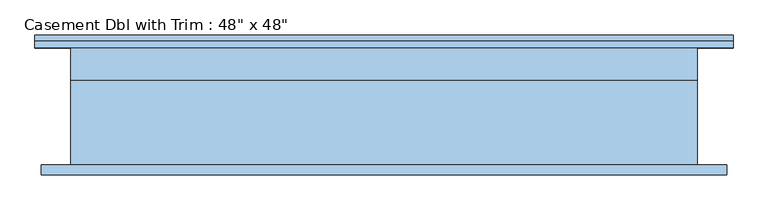
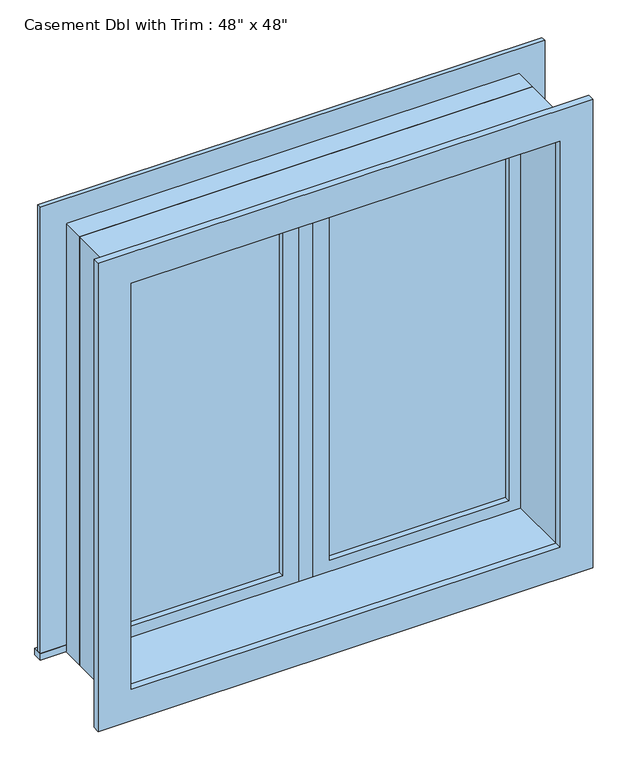
"""IFC4 building model written with IfcOpenShell, lengths in millimetres: window geometry."""

from ifc_helpers import new_model, si_unit, frame, origin, place, context, project, spatial, polyline, outline, extrude, source, transform, mapped, element, save


def window_534dcd48(model_context):
    return source(origin(), model_context, "Body", "SweptSolid", [
        extrude(outline(polyline([(63.5, 98.425), (546.1, 98.425), (546.1, 85.725), (63.5, 85.725), (63.5, 98.425)])), frame((0.0, 0.0, 977.9), z_axis=(0.0, 0.0, 1.0), x_axis=(1.0, 0.0, 0.0)), (0.0, 0.0, 1.0), 1092.2),
        extrude(outline(polyline([(2114.55, 19.05), (933.45, 19.05), (933.45, 590.55), (2114.55, 590.55), (2114.55, 19.05)]), holes=[polyline([(2070.1, 63.5), (2070.1, 546.1), (977.9, 546.1), (977.9, 63.5), (2070.1, 63.5)])]), frame((0.0, 69.85, 0.0), z_axis=(0.0, 1.0, 0.0), x_axis=(0.0, 0.0, 1.0)), (0.0, 0.0, 1.0), 44.45),
        extrude(outline(polyline([(19.05, 69.85), (-19.05, 69.85), (-19.05, 133.35), (19.05, 133.35), (19.05, 69.85)])), frame((0.0, 0.0, 933.45), z_axis=(0.0, 0.0, 1.0), x_axis=(1.0, 0.0, 0.0)), (0.0, 0.0, 1.0), 1181.1),
        extrude(outline(polyline([(-679.45, 158.75), (679.45, 158.75), (679.45, 133.35), (-679.45, 133.35), (-679.45, 158.75)])), frame((0.0, 0.0, 914.4), z_axis=(0.0, 0.0, 1.0), x_axis=(1.0, 0.0, 0.0)), (0.0, 0.0, 1.0), 19.05),
        extrude(outline(polyline([(2114.55, -590.55), (2114.55, 590.55), (933.45, 590.55), (933.45, 679.45), (2203.45, 679.45), (2203.45, -679.45), (933.45, -679.45), (933.45, -590.55), (2114.55, -590.55)])), frame((0.0, 133.35, 0.0), z_axis=(0.0, 1.0, 0.0), x_axis=(0.0, 0.0, 1.0)), (0.0, 0.0, 1.0), 12.7),
        extrude(outline(polyline([(2190.75, 666.75), (2190.75, -666.75), (857.25, -666.75), (857.25, 666.75), (2190.75, 666.75)]), holes=[polyline([(2101.85, 577.85), (946.15, 577.85), (946.15, -577.85), (2101.85, -577.85), (2101.85, 577.85)])]), frame((0.0, -114.3, 0.0), z_axis=(0.0, 1.0, 0.0), x_axis=(0.0, 0.0, 1.0)), (0.0, 0.0, 1.0), 19.05),
        extrude(outline(polyline([(-63.5, 85.725), (-546.1, 85.725), (-546.1, 98.425), (-63.5, 98.425), (-63.5, 85.725)])), frame((0.0, 0.0, 977.9), z_axis=(0.0, 0.0, 1.0), x_axis=(1.0, 0.0, 0.0)), (0.0, 0.0, 1.0), 1092.2),
        extrude(outline(polyline([(2114.55, -590.55), (933.45, -590.55), (933.45, -19.05), (2114.55, -19.05), (2114.55, -590.55)]), holes=[polyline([(2070.1, -546.1), (2070.1, -63.5), (977.9, -63.5), (977.9, -546.1), (2070.1, -546.1)])]), frame((0.0, 69.85, 0.0), z_axis=(0.0, 1.0, 0.0), x_axis=(0.0, 0.0, 1.0)), (0.0, 0.0, 1.0), 44.45),
        extrude(outline(polyline([(2133.6, -609.6), (914.4, -609.6), (914.4, 609.6), (2133.6, 609.6), (2133.6, -609.6)]), holes=[polyline([(2101.85, -577.85), (2101.85, 577.85), (946.15, 577.85), (946.15, -577.85), (2101.85, -577.85)])]), frame((0.0, -95.25, 0.0), z_axis=(0.0, 1.0, 0.0), x_axis=(0.0, 0.0, 1.0)), (0.0, 0.0, 1.0), 165.1),
        extrude(outline(polyline([(2133.6, 609.6), (2133.6, -609.6), (914.4, -609.6), (914.4, 609.6), (2133.6, 609.6)]), holes=[polyline([(2114.55, 590.55), (933.45, 590.55), (933.45, -590.55), (2114.55, -590.55), (2114.55, 590.55)])]), frame((0.0, 69.85, 0.0), z_axis=(0.0, 1.0, 0.0), x_axis=(0.0, 0.0, 1.0)), (0.0, 0.0, 1.0), 63.5),
    ])


if __name__ == "__main__":
    model = new_model("IFC4")
    model_context = context("Model", 3, world=origin())
    ifc_project = project(units=[si_unit("LENGTHUNIT", "METRE", prefix="MILLI")], contexts=[model_context])
    site = spatial("IfcSite", under=ifc_project)
    building = spatial("IfcBuilding", under=site)
    placement = place(None, origin())
    window_shape = window_534dcd48(model_context)
    element("IfcWindow", 1, ObjectType="Casement Dbl with Trim : 48\" x 48\"", at=placement, inside=building, context=model_context, shape_type="MappedRepresentation", body=[
        mapped(window_shape, transform((0.0, 0.0, 0.0), x_axis=(1.0, 0.0, 0.0), y_axis=(0.0, 1.0, 0.0), z_axis=(0.0, 0.0, 1.0))),
    ])
    save(model, "model.ifc")

# Revit data of these elements
# Type "Casement Dbl with Trim : 48\" x 48\""
#   Type Mark = "10"
#   Construction Type Id = "GSP4R"
#   Assembly Code = "B2020100"
#   Analytic Construction = "1/8 in Pilkington single glazing"
#   Visual Light Transmittance = 0.9
#   Solar Heat Gain Coefficient = 0.78
#   Heat Transfer Coefficient (U) = 0.6496 BTU/(h·ft²·°F)
#   Height = 4' - 0"
#   Default Sill Height = 3' - 0"
#   Trim Projection - Ext. = 0' - 0 1/2"
#   Trim Projection - Int. = 0' - 0 3/4"
#   Trim Width - Exterior = 0' - 3 1/2"
#   Trim Width - Interior = 0' - 3 1/2"
#   Width = 4' - 0"
#   Window Inset = 0' - 0 3/4"
#   Define Thermal Properties by = 1
#   Glass Pane Material = Glass
#   Sash Material = Glass, Clear Glazing
#   Trim Exterior Material = Earth
#   Trim Interior Material = Trim
#   Wall Closure = (empty or 0)
# Element 1 (IfcWindow, "Casement Dbl with Trim : 48\" x 48\"")
#   Materials on its faces: "Glass, Clear Glazing", "Earth", "Glass", "Trim"
# Materials
#   "Glass": class "Glass", colour RGB 0 128 192, transparency 0.75, Description = "Soda Lime Glass", Cost = 0
#   "Glass, Clear Glazing": class "Glass", colour RGB 0 128 192, transparency 0.75, Description = "Clear glazing", Cost = 0
#   "Earth": class "Generic", colour RGB 97 75 62, transparency 0, Description = "Soil", Cost = 0
#   "Trim": class "Wood", colour RGB 224 178 126, transparency 0
